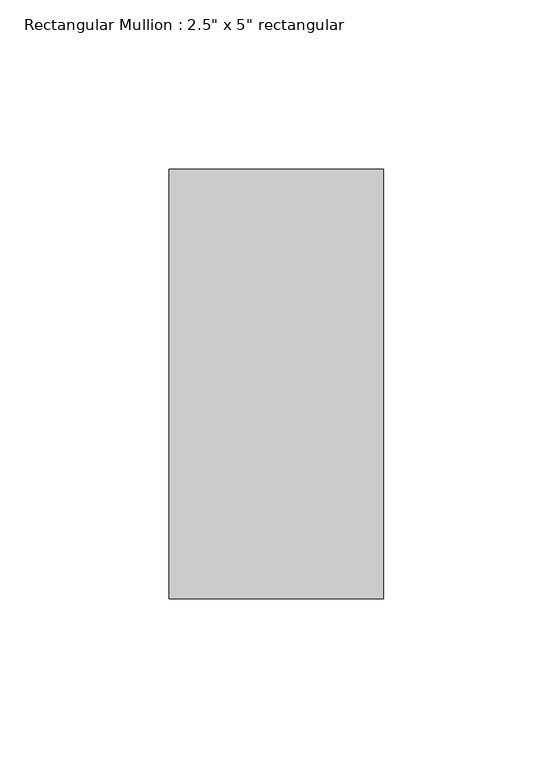
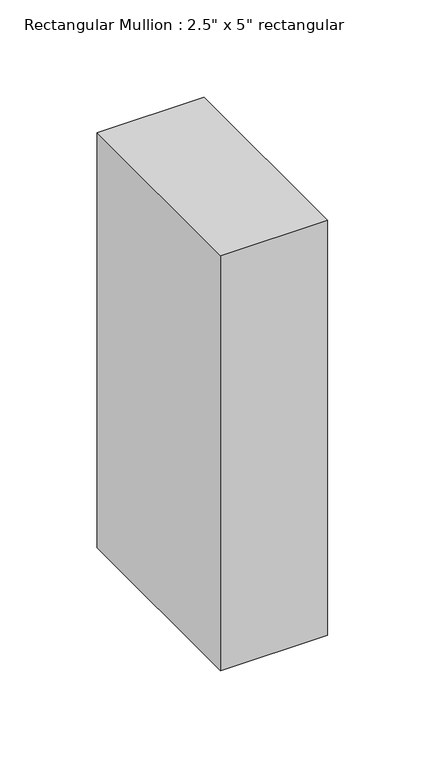
"""IFC4 building model written with IfcOpenShell, lengths in millimetres: member geometry."""

from ifc_helpers import new_model, si_unit, frame, origin, place, context, project, spatial, polyline, outline, extrude, source, transform, mapped, element, save


def member_4adcbd6e(model_context):
    return source(origin(), model_context, "Body", "SweptSolid", [
        extrude(outline(polyline([(0.0, 63.5), (0.0, -63.5), (-63.5, -63.5), (-63.5, 63.5), (0.0, 63.5)])), frame((0.0, 0.0, -260.35), z_axis=(0.0, 0.0, 1.0), x_axis=(1.0, 0.0, 0.0)), (0.0, 0.0, 1.0), 260.35),
    ])


if __name__ == "__main__":
    model = new_model("IFC4")
    model_context = context("Model", 3, world=origin())
    ifc_project = project(units=[si_unit("LENGTHUNIT", "METRE", prefix="MILLI")], contexts=[model_context])
    site = spatial("IfcSite", under=ifc_project)
    building = spatial("IfcBuilding", under=site)
    placement = place(None, origin())
    member_shape = member_4adcbd6e(model_context)
    element("IfcMember", 1, ObjectType="Rectangular Mullion : 2.5\" x 5\" rectangular", at=placement, inside=building, context=model_context, shape_type="MappedRepresentation", body=[
        mapped(member_shape, transform((0.0, 0.0, 0.0), x_axis=(1.0, 0.0, 0.0), y_axis=(0.0, 1.0, 0.0), z_axis=(0.0, 0.0, 1.0))),
    ])
    save(model, "model.ifc")

# Revit data of these elements
# Type "Rectangular Mullion : 2.5\" x 5\" rectangular"
#   built-in parameter 1007304 = 0.416667 (stored number, unit not read)
#   built-in parameter 1007301 = 0.104167 (stored number, unit not read)
#   built-in parameter 1007300 = 0.104167 (stored number, unit not read)
# Element 1 (IfcMember, "Rectangular Mullion : 2.5\" x 5\" rectangular")
#   Materials on its faces: "Aluminum"
# Materials
#   "Aluminum": class "Metal", colour RGB 247 247 247, transparency 0, Description = "Aluminum 6061", Cost = 0
